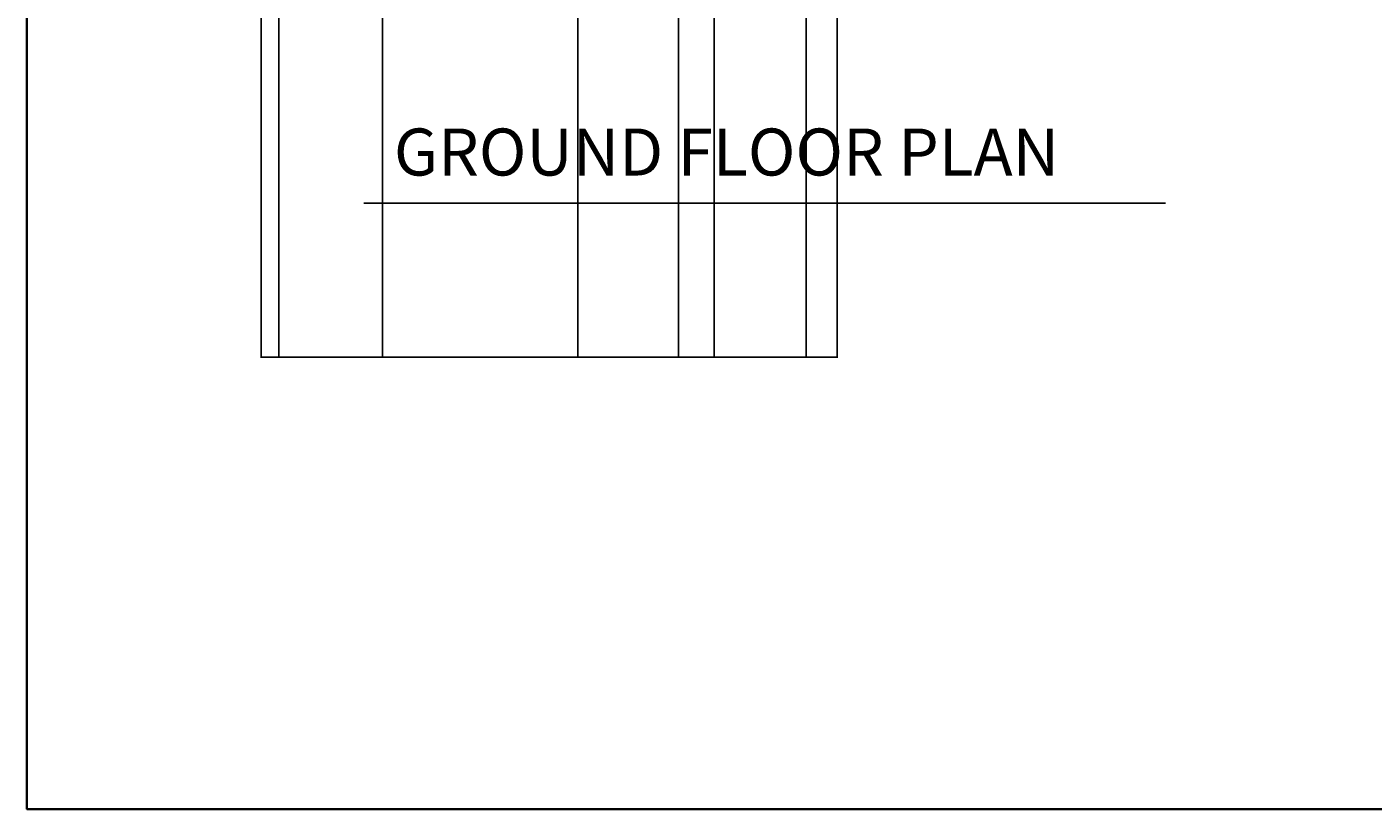
# Model space of a CAD drawing. Units: inches. Extents: x 1734 to 2405, y 1500 to 2491.
# Tile 1 of 14: x 1734 to 2078, y 1500 to 1700. Entities that reach past the tile are written whole.
import ezdxf

# ---------------------------------------------------------------- set-up
doc = ezdxf.new("R2010")
doc.units = ezdxf.units.IN
for name, color, linetype, lineweight in [('A-ANNO-DIMS', 2, 'Continuous', 18), ('A-ANNO-TITL', 7, 'Continuous', 25), ('A-ANNO-TTLB', 7, 'Continuous', 35)]:
    doc.layers.add(name, color=color, linetype=linetype, lineweight=lineweight)
doc.styles.get("Standard").update_dxf_attribs({"font": 'arial.ttf'})
doc.dimstyles.get("Standard").update_dxf_attribs({"dimtxt": 0.18, "dimasz": 0.18, "dimexe": 0.18, "dimexo": 0.0625, "dimgap": 0.09, "dimtad": 0, "dimtih": 1, "dimtoh": 1, "dimdec": 4, "dimzin": 0, "dimdsep": 46, "dimtxsty": 'Standard', "dimcen": 0.09, "dimadec": 0, "dimazin": 0, "dimtfac": 1, "dimtdec": 4, "dimtofl": 0, "dimtmove": 0, "dimatfit": 3, "dimfxl": 1, "dimtolj": 1, "dimtzin": 0, "dimarcsym": 0})

# ---------------------------------------------------------------- blocks, each defined once
blk = doc.blocks.new('*D24')
at = {"layer": 'A-ANNO-DIMS', "color": 0, "lineweight": -2, "transparency": 16777216}
for p, q in [((1793.89, 1710.7), (1793.89, 1615.47)), ((1900.39, 1710.7), (1900.39, 1615.47)), ((1794.07, 1615.65), (1846.76, 1615.65)), ((1900.21, 1615.65), (1847.53, 1615.65))]:
    blk.add_line(p, q, dxfattribs=at)
at = {"layer": 'A-ANNO-DIMS', "color": 0, "transparency": 16777216}
for points in [[(1794.07, 1615.68), (1794.07, 1615.62), (1793.89, 1615.65)], [(1900.21, 1615.68), (1900.21, 1615.62), (1900.39, 1615.65)]]:
    blk.add_solid(points, dxfattribs=at)
at = {"layer": 'Defpoints', "color": 0, "transparency": 16777216}
for p in [(1793.89, 1710.77), (1900.39, 1710.77), (1900.39, 1615.65)]:
    blk.add_point(p, dxfattribs=at)
at = {"layer": 'A-ANNO-DIMS', "color": 0, "transparency": 16777216, "insert": (1847.14, 1615.65), "char_height": 0.18, "attachment_point": 5}
blk.add_mtext('\\A1;106.5', dxfattribs=at)
blk = doc.blocks.new('*D26')
at = {"layer": 'A-ANNO-DIMS', "color": 0, "lineweight": -2, "transparency": 16777216}
for p, q in [((1900.39, 1798.76), (1900.39, 1615.47)), ((1932.99, 1798.76), (1932.99, 1615.47)), ((1900.57, 1615.65), (1916.37, 1615.65)), ((1932.81, 1615.65), (1917.02, 1615.65))]:
    blk.add_line(p, q, dxfattribs=at)
at = {"layer": 'A-ANNO-DIMS', "color": 0, "transparency": 16777216}
for points in [[(1900.57, 1615.68), (1900.57, 1615.62), (1900.39, 1615.65)], [(1932.81, 1615.68), (1932.81, 1615.62), (1932.99, 1615.65)]]:
    blk.add_solid(points, dxfattribs=at)
at = {"layer": 'Defpoints', "color": 0, "transparency": 16777216}
for p in [(1900.39, 1798.82), (1932.99, 1798.82), (1932.99, 1615.65)]:
    blk.add_point(p, dxfattribs=at)
at = {"layer": 'A-ANNO-DIMS', "color": 0, "transparency": 16777216, "insert": (1916.69, 1615.65), "char_height": 0.18, "attachment_point": 5}
blk.add_mtext('\\A1;32.6', dxfattribs=at)
blk = doc.blocks.new('*D32')
at = {"layer": 'A-ANNO-DIMS', "color": 0, "lineweight": -2, "transparency": 16777216}
for p, q in [((1798.39, 2202.26), (1798.39, 1615.47)), ((1824.83, 2202.26), (1824.83, 1615.47)), ((1798.57, 1615.65), (1811.22, 1615.65)), ((1824.65, 1615.65), (1812.01, 1615.65))]:
    blk.add_line(p, q, dxfattribs=at)
at = {"layer": 'A-ANNO-DIMS', "color": 0, "transparency": 16777216}
for points in [[(1798.57, 1615.68), (1798.57, 1615.62), (1798.39, 1615.65)], [(1824.65, 1615.68), (1824.65, 1615.62), (1824.83, 1615.65)]]:
    blk.add_solid(points, dxfattribs=at)
at = {"layer": 'Defpoints', "color": 0, "transparency": 16777216}
for p in [(1798.39, 2202.32), (1824.83, 2202.32), (1824.83, 1615.65)]:
    blk.add_point(p, dxfattribs=at)
at = {"layer": 'A-ANNO-DIMS', "color": 0, "transparency": 16777216, "insert": (1811.61, 1615.65), "char_height": 0.18, "attachment_point": 5}
blk.add_mtext('\\A1;26.44', dxfattribs=at)
blk = doc.blocks.new('*D33')
at = {"layer": 'A-ANNO-DIMS', "color": 0, "lineweight": -2, "transparency": 16777216}
for p, q in [((1824.83, 2202.26), (1824.83, 1615.47)), ((1874.68, 2202.26), (1874.68, 1615.47)), ((1825.01, 1615.65), (1849.36, 1615.65)), ((1874.5, 1615.65), (1850.15, 1615.65))]:
    blk.add_line(p, q, dxfattribs=at)
at = {"layer": 'A-ANNO-DIMS', "color": 0, "transparency": 16777216}
for points in [[(1825.01, 1615.68), (1825.01, 1615.62), (1824.83, 1615.65)], [(1874.5, 1615.68), (1874.5, 1615.62), (1874.68, 1615.65)]]:
    blk.add_solid(points, dxfattribs=at)
at = {"layer": 'Defpoints', "color": 0, "transparency": 16777216}
for p in [(1824.83, 2202.32), (1874.68, 2202.32), (1874.68, 1615.65)]:
    blk.add_point(p, dxfattribs=at)
at = {"layer": 'A-ANNO-DIMS', "color": 0, "transparency": 16777216, "insert": (1849.76, 1615.65), "char_height": 0.18, "attachment_point": 5}
blk.add_mtext('\\A1;49.84', dxfattribs=at)
blk = doc.blocks.new('*D34')
at = {"layer": 'A-ANNO-DIMS', "color": 0, "lineweight": -2, "transparency": 16777216}
for p, q in [((1909.52, 2202.26), (1909.52, 1615.47)), ((1940.89, 2204.68), (1940.89, 1615.47)), ((1909.7, 1615.65), (1924.81, 1615.65)), ((1940.71, 1615.65), (1925.6, 1615.65))]:
    blk.add_line(p, q, dxfattribs=at)
at = {"layer": 'A-ANNO-DIMS', "color": 0, "transparency": 16777216}
for points in [[(1909.7, 1615.68), (1909.7, 1615.62), (1909.52, 1615.65)], [(1940.71, 1615.68), (1940.71, 1615.62), (1940.89, 1615.65)]]:
    blk.add_solid(points, dxfattribs=at)
at = {"layer": 'Defpoints', "color": 0, "transparency": 16777216}
for p in [(1909.52, 2202.32), (1940.89, 2204.75), (1940.89, 1615.65)]:
    blk.add_point(p, dxfattribs=at)
at = {"layer": 'A-ANNO-DIMS', "color": 0, "transparency": 16777216, "insert": (1925.21, 1615.65), "char_height": 0.18, "attachment_point": 5}
blk.add_mtext('\\A1;31.37', dxfattribs=at)

msp = doc.modelspace()

# ---------------------------------------------------------------- linework, layer by layer
at = {"layer": 'A-ANNO-TITL'}
msp.add_line((1820.0714, 1654.9968), (2024.6456, 1654.9968), dxfattribs=at)
at = {"layer": 'A-ANNO-TTLB'}
msp.add_lwpolyline([(1734.1307, 2491.1293), (2404.5589, 2491.1293), (2404.5589, 1500.293), (1734.1307, 1500.293)], close=True, dxfattribs=at)

# ---------------------------------------------------------------- texts
at = {"layer": 'A-ANNO-TITL', "insert": (1827.7799, 1674.0229), "char_height": 12, "attachment_point": 1}
msp.add_mtext_dynamic_manual_height_columns('GROUND FLOOR PLAN ', width=211.533087, gutter_width=12.5, heights=[0], dxfattribs=at)

# ---------------------------------------------------------------- dimensions: what is measured, and where the dimension line sits
at = {"layer": 'A-ANNO-DIMS'}
for base, p1, p2, override, picture, middle in [((1824.8343, 1615.6468), (1798.3942, 2202.3246), (1824.8343, 2202.3246), {"dimdec": 2, "dimlfac": 1, "dimrnd": 0, "dimzin": 0, "dimdsep": 46, "dimlunit": 2}, '*D32', (1811.6142, 1615.6468)), ((1874.676, 1615.6468), (1824.8343, 2202.3246), (1874.676, 2202.3246), {"dimdec": 2, "dimlfac": 1, "dimrnd": 0, "dimzin": 0, "dimdsep": 46, "dimlunit": 2}, '*D33', (1849.7551, 1615.6468)), ((1940.8942, 1615.6468), (1909.5222, 2202.3246), (1940.8942, 2204.7456), {"dimdec": 2, "dimlfac": 1, "dimrnd": 0, "dimzin": 0, "dimdsep": 46, "dimlunit": 2}, '*D34', (1925.2082, 1615.6468)), ((1932.9923, 1615.6468), (1900.3942, 1798.8246), (1932.9923, 1798.8246), {"dimdec": 1, "dimlfac": 1, "dimrnd": 0, "dimzin": 0, "dimdsep": 46, "dimlunit": 2}, '*D26', (1916.6932, 1615.6468)), ((1900.3942, 1615.6468), (1793.8942, 1710.7667), (1900.3942, 1710.7667), {"dimdec": 1, "dimlfac": 1, "dimrnd": 0, "dimzin": 0, "dimdsep": 46, "dimlunit": 2}, '*D24', (1847.1442, 1615.6468))]:
    dim = msp.add_linear_dim(base=base, p1=p1, p2=p2, dimstyle='Standard', override=override, dxfattribs=at)
    dim.commit()
    dim.dimension.update_dxf_attribs({"geometry": picture, "text_midpoint": middle})

doc.saveas('drawing.dxf')
